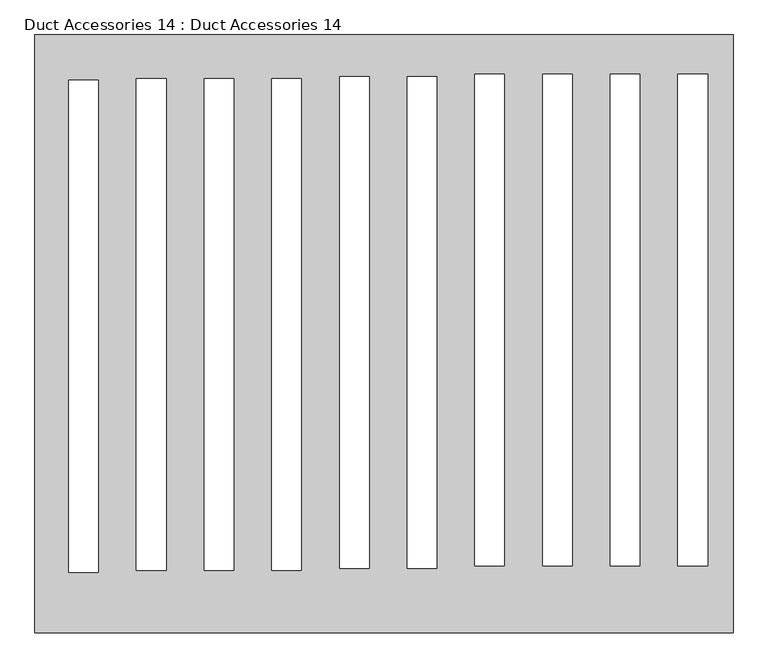
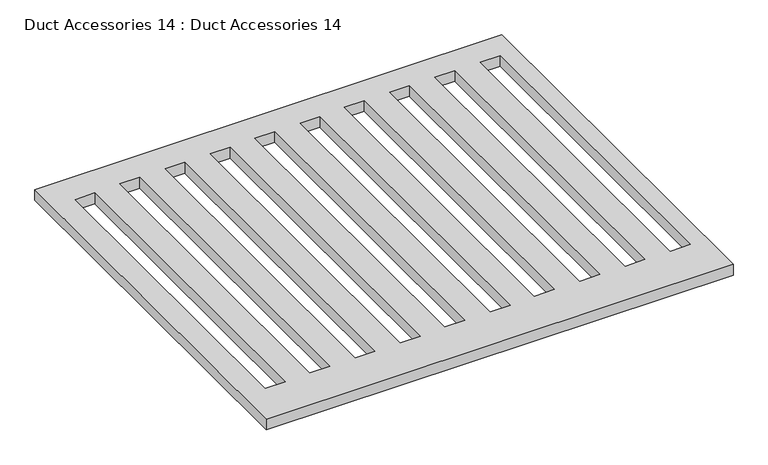
"""IFC4 building model written with IfcOpenShell, lengths in millimetres: damper geometry, Duct Accessories 14 : Duct Accessories 14."""

from ifc_helpers import new_model, si_unit, frame, origin, place, context, project, spatial, polyline, outline, extrude, source, transform, mapped, element, save


def duct_accessories_14_duct_accessories_14_a27dce4f(model_context):
    return source(origin(), model_context, "Body", "SweptSolid", [
        extrude(outline(polyline([(-3622.597125, 4711.0719226), (-3622.597125, -676.0934478), (-9909.097125, -676.0934478), (-9909.097125, 4711.0719226), (-3622.597125, 4711.0719226)]), holes=[polyline([(-9337.597125, 4302.3065522), (-9604.297125, 4302.3065522), (-9604.297125, -129.9934478), (-9337.597125, -129.9934478), (-9337.597125, 4302.3065522)]), polyline([(-8728.1713452, 4316.8797774), (-8994.8713452, 4316.8797774), (-8994.8713452, -115.4202226), (-8728.1713452, -115.4202226), (-8728.1713452, 4316.8797774)]), polyline([(-8118.5713452, 4316.8797774), (-8385.2713452, 4316.8797774), (-8385.2713452, -115.4202226), (-8118.5713452, -115.4202226), (-8118.5713452, 4316.8797774)]), polyline([(-7508.9713452, 4316.8797774), (-7775.6713452, 4316.8797774), (-7775.6713452, -115.4202226), (-7508.9713452, -115.4202226), (-7508.9713452, 4316.8797774)]), polyline([(-6899.6674051, 4335.8763206), (-7166.3674051, 4335.8763206), (-7166.3674051, -96.4236794), (-6899.6674051, -96.4236794), (-6899.6674051, 4335.8763206)]), polyline([(-6290.0674051, 4335.8763206), (-6556.7674051, 4335.8763206), (-6556.7674051, -96.4236794), (-6290.0674051, -96.4236794), (-6290.0674051, 4335.8763206)]), polyline([(-5680.9065671, 4359.0114319), (-5947.6065671, 4359.0114319), (-5947.6065671, -73.2885681), (-5680.9065671, -73.2885681), (-5680.9065671, 4359.0114319)]), polyline([(-5071.3065671, 4359.0114319), (-5338.0065671, 4359.0114319), (-5338.0065671, -73.2885681), (-5071.3065671, -73.2885681), (-5071.3065671, 4359.0114319)]), polyline([(-4461.7065671, 4359.0114319), (-4728.4065671, 4359.0114319), (-4728.4065671, -73.2885681), (-4461.7065671, -73.2885681), (-4461.7065671, 4359.0114319)]), polyline([(-3852.1065671, 4359.0114319), (-4118.8065671, 4359.0114319), (-4118.8065671, -73.2885681), (-3852.1065671, -73.2885681), (-3852.1065671, 4359.0114319)])]), frame((0.0, 0.0, 44805.6), z_axis=(0.0, 0.0, 1.0), x_axis=(1.0, 0.0, 0.0)), (0.0, 0.0, 1.0), 152.4),
    ])


if __name__ == "__main__":
    model = new_model("IFC4")
    model_context = context("Model", 3, world=origin())
    ifc_project = project(units=[si_unit("LENGTHUNIT", "METRE", prefix="MILLI")], contexts=[model_context])
    site = spatial("IfcSite", under=ifc_project)
    building = spatial("IfcBuilding", under=site)
    placement = place(None, origin())
    duct_accessories_14_duct_accessories_14_shape = duct_accessories_14_duct_accessories_14_a27dce4f(model_context)
    element("IfcDamper", 1, ObjectType="Duct Accessories 14 : Duct Accessories 14", at=placement, inside=building, context=model_context, shape_type="MappedRepresentation", body=[
        mapped(duct_accessories_14_duct_accessories_14_shape, transform((0.0, 0.0, 0.0), x_axis=(1.0, 0.0, 0.0), y_axis=(0.0, 1.0, 0.0), z_axis=(0.0, 0.0, 1.0))),
    ])
    save(model, "model.ifc")

# Revit data of these elements
# Element 1 (IfcDamper, "Duct Accessories 14 : Duct Accessories 14")
#   Materials on its faces: "Clad - White"
# Materials
#   "Clad - White": class "Wood", colour RGB 242 242 238, transparency 0, Cost = 0
